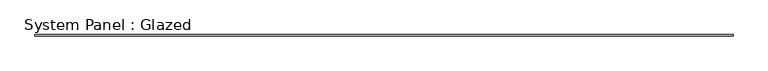
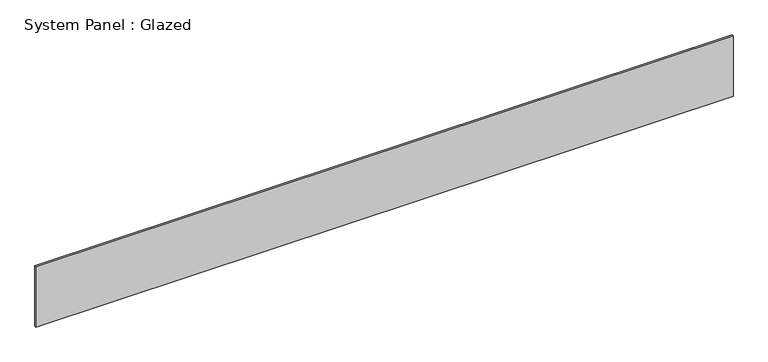
"""IFC4 building model written with IfcOpenShell, lengths in millimetres: plate geometry, System Panel : Glazed."""

from ifc_helpers import new_model, si_unit, origin, origin_with_axes, place, context, project, spatial, polyline, outline, extrude, source, transform, mapped, element, save


def system_panel_glazed_8d5a176b(model_context):
    return source(origin(), model_context, "Body", "SweptSolid", [
        extrude(outline(polyline([(6309.5276373, 19.05), (-6309.5276373, 19.05), (-6309.5276373, 44.45), (6309.5276373, 44.45), (6309.5276373, 19.05)])), origin_with_axes(), (0.0, 0.0, 1.0), 1155.7),
    ])


if __name__ == "__main__":
    model = new_model("IFC4")
    model_context = context("Model", 3, world=origin())
    ifc_project = project(units=[si_unit("LENGTHUNIT", "METRE", prefix="MILLI")], contexts=[model_context])
    site = spatial("IfcSite", under=ifc_project)
    building = spatial("IfcBuilding", under=site)
    placement = place(None, origin())
    system_panel_glazed_shape = system_panel_glazed_8d5a176b(model_context)
    element("IfcPlate", 1, ObjectType="System Panel : Glazed", at=placement, inside=building, context=model_context, shape_type="MappedRepresentation", body=[
        mapped(system_panel_glazed_shape, transform((0.0, 0.0, 0.0), x_axis=(1.0, 0.0, 0.0), y_axis=(0.0, 1.0, 0.0), z_axis=(0.0, 0.0, 1.0))),
    ])
    save(model, "model.ifc")

# Revit data of these elements
# Type "System Panel : Glazed"
#   Construction Type Id = "GSP4R"
#   Analytic Construction = "1/8 in Pilkington single glazing"
#   Visual Light Transmittance = 0.9
#   Solar Heat Gain Coefficient = 0.86
#   Heat Transfer Coefficient (U) = 1.18115 BTU/(h·ft²·°F)
# Element 1 (IfcPlate, "System Panel : Glazed")
#   Materials on its faces: "Glass"
# Materials
#   "Glass": class "Glass", colour RGB 0 128 192, transparency 0.75, Description = "Soda Lime Glass", Cost = 0
